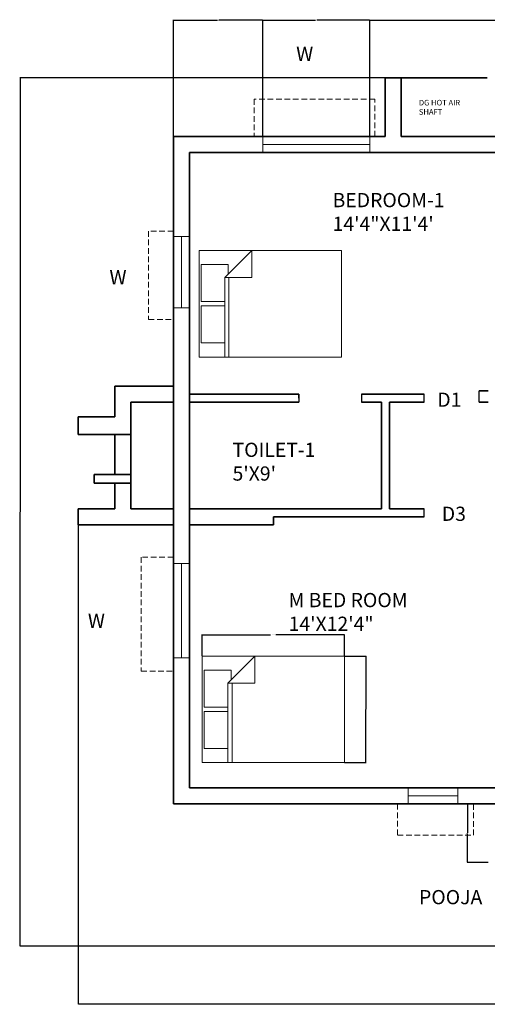
# Model space of a CAD drawing. Units: inches. Extents: x 514 to 1200, y -110 to 470.
# Tile 1 of 3: x 514 to 777, y -84 to 470. Entities that reach past the tile are written whole.
import ezdxf

# ---------------------------------------------------------------- set-up
doc = ezdxf.new("R2010")
doc.units = ezdxf.units.IN
doc.linetypes.add('HIDDEN2', pattern=[4.7625, 3.175, -1.5875])
for name, color, linetype, lineweight in [('A-ANNO-DIMS', 2, 'Continuous', 18), ('A-ANNO-IDEN', 3, 'Continuous', 18), ('A-AREA-IDEN', 7, 'Continuous', 18), ('A-DOOR', 3, 'Continuous', 25), ('A-FLOR-OVHD', 8, 'HIDDEN2', 18), ('A-FURN', 8, 'Continuous', 18), ('A-GLAZ', 4, 'Continuous', 18), ('A-WALL', 7, 'Continuous', 35)]:
    doc.layers.add(name, color=color, linetype=linetype, lineweight=lineweight)
doc.dimstyles.get("Standard").update_dxf_attribs({"dimtxt": 0.18, "dimasz": 0.18, "dimexe": 0.18, "dimexo": 0.0625, "dimgap": 0.09, "dimtad": 0, "dimtih": 1, "dimtoh": 1, "dimdec": 4, "dimzin": 0, "dimdsep": 46, "dimtxsty": 'Standard', "dimcen": 0.09, "dimadec": 0, "dimazin": 0, "dimtfac": 1, "dimtdec": 4, "dimtofl": 0, "dimtmove": 0, "dimatfit": 3, "dimfxl": 1, "dimtolj": 1, "dimtzin": 0, "dimarcsym": 0})

# ---------------------------------------------------------------- blocks, each defined once
blk = doc.blocks.new('Bed - Queen')
for p, q in [((0, -80.00003), (0, 0)), ((0, 0), (59.99999, 0)), ((59.99999, 0), (59.99999, -80.00003)), ((7.99999, -1.2), (28.79998, -1.2)), ((7.99999, -14.4), (7.99999, -1.2)), ((28.79998, -1.2), (28.79998, -14.4)), ((31.19999, -1.2), (51.99999, -1.2)), ((31.19999, -14.4), (31.19999, -1.2)), ((51.99999, -1.2), (51.99999, -16.4)), ((0, -14.4), (44.8, -14.4)), ((59.99999, -29.6), (44.8, -14.4)), ((44.8, -14.4), (44.8, -29.6)), ((51.99999, -16.4), (46.79936, -16.4)), ((44.8, -16.8), (0, -16.8)), ((44.8, -29.6), (59.99999, -29.6)), ((59.99999, -80.00003), (0, -80.00003))]:
    blk.add_line(p, q)
blk = doc.blocks.new('*D14')
at = {"layer": 'A-ANNO-DIMS', "color": 0, "lineweight": -2, "transparency": 16777216}
for p, q in [((617.04, 112.31), (617.04, 124.43)), ((617.22, 124.25), (655.52, 124.25)), ((696.86, 124.25), (658.55, 124.25)), ((697.04, 112.31), (697.04, 124.43))]:
    blk.add_line(p, q, dxfattribs=at)
at = {"layer": 'A-ANNO-DIMS', "color": 0, "transparency": 16777216}
for points in [[(617.22, 124.28), (617.22, 124.22), (617.04, 124.25)], [(696.86, 124.28), (696.86, 124.22), (697.04, 124.25)]]:
    blk.add_solid(points, dxfattribs=at)
at = {"layer": 'Defpoints', "color": 0, "transparency": 16777216}
for p in [(617.04, 124.25), (617.04, 112.25), (697.04, 112.25)]:
    blk.add_point(p, dxfattribs=at)
at = {"layer": 'A-ANNO-DIMS', "color": 0, "transparency": 16777216, "insert": (657.04, 124.25), "char_height": 0.18, "attachment_point": 5}
blk.add_mtext('\\A1;QUEEN BED 80 TYP.', dxfattribs=at)
blk = doc.blocks.new('*D15')
at = {"layer": 'A-ANNO-DIMS', "color": 0, "lineweight": -2, "transparency": 16777216}
for p, q in [((697.1, 112.25), (709.22, 112.25)), ((709.04, 112.07), (709.04, 82.43)), ((709.04, 52.43), (709.04, 82.07)), ((697.1, 52.25), (709.22, 52.25))]:
    blk.add_line(p, q, dxfattribs=at)
at = {"layer": 'A-ANNO-DIMS', "color": 0, "transparency": 16777216}
for points in [[(709.01, 112.07), (709.07, 112.07), (709.04, 112.25)], [(709.01, 52.43), (709.07, 52.43), (709.04, 52.25)]]:
    blk.add_solid(points, dxfattribs=at)
at = {"layer": 'Defpoints', "color": 0, "transparency": 16777216}
for p in [(697.04, 112.25), (709.04, 112.25), (697.04, 52.25)]:
    blk.add_point(p, dxfattribs=at)
at = {"layer": 'A-ANNO-DIMS', "color": 0, "transparency": 16777216, "insert": (709.04, 82.25), "char_height": 0.18, "attachment_point": 5}
blk.add_mtext('\\A1;60 TYP.', dxfattribs=at)
blk = doc.blocks.new('*D17')
at = {"layer": 'A-ANNO-DIMS', "color": 0, "lineweight": -2, "transparency": 16777216}
for p, q in [((777.83, 29.02), (766.01, 29.02)), ((766.19, 28.84), (766.19, 12.7)), ((766.19, -3.8), (766.19, 12.34)), ((777.83, -3.98), (766.01, -3.98))]:
    blk.add_line(p, q, dxfattribs=at)
at = {"layer": 'A-ANNO-DIMS', "color": 0, "transparency": 16777216}
for points in [[(766.16, 28.84), (766.22, 28.84), (766.19, 29.02)], [(766.16, -3.8), (766.22, -3.8), (766.19, -3.98)]]:
    blk.add_solid(points, dxfattribs=at)
at = {"layer": 'Defpoints', "color": 0, "transparency": 16777216}
for p in [(766.19, 29.02), (777.89, 29.02), (777.89, -3.98)]:
    blk.add_point(p, dxfattribs=at)
at = {"layer": 'A-ANNO-DIMS', "color": 0, "transparency": 16777216, "insert": (766.19, 12.52), "char_height": 0.18, "attachment_point": 5}
blk.add_mtext('\\A1;33 TYP.', dxfattribs=at)
blk = doc.blocks.new('*D24')
at = {"layer": 'A-ANNO-DIMS', "color": 0, "lineweight": -2, "transparency": 16777216}
for p, q in [((600.890564, 404.583196), (600.890564, 470.250696)), ((601.070564, 470.070696), (625.592556, 470.070696)), ((650.924548, 470.070696), (626.402556, 470.070696)), ((651.104548, 404.583196), (651.104548, 470.250696))]:
    blk.add_line(p, q, dxfattribs=at)
at = {"layer": 'A-ANNO-DIMS', "color": 0, "transparency": 16777216}
for points in [[(601.070564, 470.100696), (601.070564, 470.040696), (600.890564, 470.070696)], [(650.924548, 470.100696), (650.924548, 470.040696), (651.104548, 470.070696)]]:
    blk.add_solid(points, dxfattribs=at)
at = {"layer": 'Defpoints', "color": 0, "transparency": 16777216}
for p in [(651.104548, 470.070696), (600.890564, 404.520696), (651.104548, 404.520696)]:
    blk.add_point(p, dxfattribs=at)
at = {"layer": 'A-ANNO-DIMS', "color": 0, "transparency": 16777216, "insert": (625.997556, 470.070696), "char_height": 0.18, "attachment_point": 5}
blk.add_mtext('\\A1;50.21', dxfattribs=at)
blk = doc.blocks.new('*D25')
at = {"layer": 'A-ANNO-DIMS', "color": 0, "lineweight": -2, "transparency": 16777216}
for p, q in [((651.1, 404.58), (651.1, 470.25)), ((651.28, 470.07), (680.79, 470.07)), ((711.1, 470.07), (681.6, 470.07)), ((711.28, 404.58), (711.28, 470.25))]:
    blk.add_line(p, q, dxfattribs=at)
at = {"layer": 'A-ANNO-DIMS', "color": 0, "transparency": 16777216}
for points in [[(651.28, 470.1), (651.28, 470.04), (651.1, 470.07)], [(711.1, 470.1), (711.1, 470.04), (711.28, 470.07)]]:
    blk.add_solid(points, dxfattribs=at)
at = {"layer": 'Defpoints', "color": 0, "transparency": 16777216}
for p in [(711.28, 470.07), (651.1, 404.52), (711.28, 404.52)]:
    blk.add_point(p, dxfattribs=at)
at = {"layer": 'A-ANNO-DIMS', "color": 0, "transparency": 16777216, "insert": (681.19, 470.07), "char_height": 0.18, "attachment_point": 5}
blk.add_mtext('\\A1;60.18', dxfattribs=at)
blk = doc.blocks.new('*D26')
at = {"layer": 'A-ANNO-DIMS', "color": 0, "lineweight": -2, "transparency": 16777216}
for p, q in [((711.28, 404.58), (711.28, 470.25)), ((711.46, 470.07), (797.69, 470.07)), ((884.94, 470.07), (798.71, 470.07)), ((885.12, 404.58), (885.12, 470.25))]:
    blk.add_line(p, q, dxfattribs=at)
at = {"layer": 'A-ANNO-DIMS', "color": 0, "transparency": 16777216}
for points in [[(711.46, 470.1), (711.46, 470.04), (711.28, 470.07)], [(884.94, 470.1), (884.94, 470.04), (885.12, 470.07)]]:
    blk.add_solid(points, dxfattribs=at)
at = {"layer": 'Defpoints', "color": 0, "transparency": 16777216}
for p in [(885.12, 470.07), (711.28, 404.52), (885.12, 404.52)]:
    blk.add_point(p, dxfattribs=at)
at = {"layer": 'A-ANNO-DIMS', "color": 0, "transparency": 16777216, "insert": (798.2, 470.07), "char_height": 0.18, "attachment_point": 5}
blk.add_mtext('\\A1;173.83', dxfattribs=at)
blk = doc.blocks.new('*D36')
at = {"layer": 'A-ANNO-DIMS', "color": 0, "lineweight": -2, "transparency": 16777216}
for p, q in [((1166.99, 243.01), (1166.99, -83.71)), ((547.32, 185.96), (547.32, -83.71)), ((547.5, -83.53), (856.73, -83.53)), ((1166.81, -83.53), (857.57, -83.53))]:
    blk.add_line(p, q, dxfattribs=at)
at = {"layer": 'A-ANNO-DIMS', "color": 0, "transparency": 16777216}
for points in [[(547.5, -83.5), (547.5, -83.56), (547.32, -83.53)], [(1166.81, -83.5), (1166.81, -83.56), (1166.99, -83.53)]]:
    blk.add_solid(points, dxfattribs=at)
at = {"layer": 'Defpoints', "color": 0, "transparency": 16777216}
for p in [(1166.99, 243.07), (547.32, 186.02), (1166.99, -83.53)]:
    blk.add_point(p, dxfattribs=at)
at = {"layer": 'A-ANNO-DIMS', "color": 0, "transparency": 16777216, "insert": (857.15, -83.53), "char_height": 0.18, "attachment_point": 5}
blk.add_mtext('\\A1;619.7', dxfattribs=at)
blk = doc.blocks.new('*D37')
at = {"layer": 'A-ANNO-DIMS', "color": 0, "lineweight": -2, "transparency": 16777216}
for p, q in [((719.82324, 437.520696), (514.588716, 437.520696)), ((514.768716, 437.340696), (514.768716, 193.450696)), ((514.768716, -50.799304), (514.768716, 193.090696)), ((846.828064, -50.979304), (514.588716, -50.979304))]:
    blk.add_line(p, q, dxfattribs=at)
at = {"layer": 'A-ANNO-DIMS', "color": 0, "transparency": 16777216}
for points in [[(514.738716, 437.340696), (514.798716, 437.340696), (514.768716, 437.520696)], [(514.738716, -50.799304), (514.798716, -50.799304), (514.768716, -50.979304)]]:
    blk.add_solid(points, dxfattribs=at)
at = {"layer": 'Defpoints', "color": 0, "transparency": 16777216}
for p in [(514.768716, 437.520696), (719.88574, 437.520696), (846.890564, -50.979304)]:
    blk.add_point(p, dxfattribs=at)
at = {"layer": 'A-ANNO-DIMS', "color": 0, "transparency": 16777216, "insert": (514.768716, 193.270696), "char_height": 0.18, "attachment_point": 5}
blk.add_mtext('\\A1;488.5', dxfattribs=at)

msp = doc.modelspace()

# ---------------------------------------------------------------- linework, layer by layer
at = {"layer": 'A-DOOR'}
for p, q in [((772.9065, 255.0207), (772.9065, 261.4252)), ((671.3734, 257.2707), (671.3734, 259.5207)), ((671.3734, 259.5207), (671.3734, 255.0207)), ((706.6585, 259.5207), (706.6585, 255.0207)), ((741.8906, 255.0207), (741.8906, 259.5207)), ((741.8906, 190.5207), (741.8906, 195.0207))]:
    msp.add_line(p, q, dxfattribs=at)
at = {"layer": 'A-FLOR-OVHD'}
for p, q in [((714.1676, 425.5708), (646.3079, 425.5708)), ((646.3079, 425.5708), (646.3079, 404.5207)), ((714.1676, 404.5207), (714.1676, 425.5708)), ((600.8906, 351.2891), (586.9342, 351.2891)), ((586.9342, 351.2891), (586.9342, 301.4805)), ((586.9342, 301.4805), (600.8906, 301.4805)), ((600.8906, 167.7812), (582.8053, 167.7812)), ((582.8053, 167.7812), (582.8053, 103.6598)), ((582.8053, 103.6598), (600.8906, 103.6598)), ((726.9376, 29.0207), (726.9376, 11.4444)), ((769.6276, 11.4444), (769.6276, 29.0207)), ((726.9376, 11.4444), (769.6276, 11.4444))]:
    msp.add_line(p, q, dxfattribs=at)
at = {"layer": 'A-GLAZ'}
for p, q in [((651.1045, 404.5207), (651.1045, 395.5207)), ((711.283, 400.0207), (711.283, 404.5207)), ((711.283, 404.5207), (711.283, 395.5207)), ((651.1045, 395.5207), (651.1045, 400.0207)), ((651.1045, 400.0207), (711.283, 400.0207)), ((600.8906, 348.2213), (609.8906, 348.2213)), ((609.8906, 348.2213), (605.3906, 348.2213)), ((605.3906, 348.2213), (605.3906, 308.2207)), ((605.3906, 308.2207), (600.8906, 308.2207)), ((600.8906, 308.2207), (609.8906, 308.2207)), ((600.8906, 164.3544), (609.8906, 164.3544)), ((609.8906, 164.3544), (605.3906, 164.3544)), ((605.3906, 164.3544), (605.3906, 111.1618)), ((605.3906, 111.1618), (600.8906, 111.1618)), ((600.8906, 111.1618), (609.8906, 111.1618)), ((732.8501, 38.0207), (732.8501, 29.0207)), ((732.8501, 29.0207), (732.8501, 33.5207)), ((732.8501, 33.5207), (760.8245, 33.5207)), ((760.8245, 33.5207), (760.8245, 38.0207)), ((760.8245, 38.0207), (760.8245, 29.0207))]:
    msp.add_line(p, q, dxfattribs=at)
at = {"layer": 'A-WALL'}
for p, q in [((719.8857, 437.5207), (719.8857, 404.5207)), ((728.8857, 437.5207), (719.8857, 437.5207)), ((777.3906, 437.5207), (728.8857, 437.5207)), ((728.8857, 437.5207), (728.8857, 404.5207)), ((600.8906, 404.5207), (719.8857, 404.5207)), ((600.8906, 29.0207), (600.8906, 404.5207)), ((728.8857, 404.5207), (1142.8906, 404.5207)), ((609.8906, 395.5207), (781.8906, 395.5207)), ((609.8906, 38.0207), (609.8906, 395.5207)), ((567.8906, 264.0207), (567.8906, 246.7778)), ((600.8906, 264.0207), (567.8906, 264.0207)), ((772.9065, 261.4252), (777.8906, 261.4252)), ((600.8906, 255.0207), (576.8906, 255.0207)), ((576.8906, 255.0207), (576.8906, 195.0207)), ((609.8906, 259.5207), (671.3734, 259.5207)), ((609.8906, 259.5207), (671.3734, 259.5207)), ((609.8906, 255.0207), (671.3734, 255.0207)), ((609.8906, 255.0207), (671.3734, 255.0207)), ((706.6585, 259.5207), (741.8906, 259.5207)), ((706.6585, 259.5207), (741.8906, 259.5207)), ((706.6585, 255.0207), (717.8906, 255.0207)), ((706.6585, 255.0207), (717.8906, 255.0207)), ((717.8906, 195.0207), (717.8906, 255.0207)), ((722.3906, 195.0207), (722.3906, 255.0207)), ((722.3906, 255.0207), (741.8906, 255.0207)), ((722.3906, 255.0207), (741.8906, 255.0207)), ((777.8906, 255.0207), (772.9065, 255.0207)), ((547.3187, 236.9335), (547.3187, 246.7778)), ((547.3187, 246.7778), (567.8906, 246.7778)), ((576.8906, 236.9335), (547.3187, 236.9335)), ((567.8906, 236.9335), (567.8906, 214.3425)), ((576.8906, 214.3425), (556.4172, 214.3425)), ((556.4172, 214.3425), (556.4172, 209.4406)), ((556.4172, 209.4406), (576.8906, 209.4406)), ((567.8906, 209.4406), (567.8906, 195.0207)), ((547.3187, 186.0207), (547.3187, 195.0207)), ((547.3187, 195.0207), (567.8906, 195.0207)), ((576.8906, 195.0207), (600.8906, 195.0207)), ((609.8906, 195.0207), (717.8906, 195.0207)), ((722.3906, 195.0207), (741.8906, 195.0207)), ((657.1918, 186.0207), (657.1918, 190.5207)), ((657.1918, 190.5207), (722.3906, 190.5207)), ((657.1918, 190.5207), (741.8906, 190.5207)), ((567.8906, 186.0207), (547.3187, 186.0207)), ((567.8906, 186.0207), (600.8906, 186.0207)), ((609.8906, 186.0207), (657.1918, 186.0207)), ((609.8906, 38.0207), (983.8906, 38.0207)), ((600.8906, 29.0207), (983.8906, 29.0207))]:
    msp.add_line(p, q, dxfattribs=at)

# ---------------------------------------------------------------- block references
at = {"layer": 'A-FURN', "rotation": 90}
for p in [(615.3484, 280.4737), (617.0399, 52.2514)]:
    msp.add_blockref('Bed - Queen', p, dxfattribs=at)

# ---------------------------------------------------------------- texts
at = {"layer": 'A-ANNO-IDEN', "char_height": 8, "attachment_point": 1}
for s, insert in [('{\\fTimes New Roman|b0|i0|c0|p18;W}', (669.9162, 455.055)), ('{\\fTimes New Roman|b0|i0|c0|p18;W}', (564.9379, 329.3302)), ('{\\fTimes New Roman|b0|i0|c0|p18;D1}', (749.2884, 260.4506)), ('\\pxt2;{\\fTimes New Roman|b0|i0|c0|p18;D3}', (751.8117, 196.2713)), ('{\\fTimes New Roman|b0|i0|c0|p18;W}', (552.8049, 136.0875))]:
    msp.add_mtext_dynamic_manual_height_columns(s, width=92.773282, gutter_width=12.5, heights=[0], dxfattribs=dict(at, insert=insert))
at = {"layer": 'A-AREA-IDEN', "attachment_point": 1}
for s, width, gutter_width, insert, char_height in [('{\\fTimes New Roman|b0|i0|c0|p18;DG HOT AIR SHAFT}', 36.387649, 4.9028, (738.9027, 425.1429), 3.13777), ('{\\fTimes New Roman|b0|i0|c0|p18;BEDROOM-1\\P14\'4"X11\'4\'}', 92.773282, 12.5, (690.384, 372.7481), 8), ("{\\fTimes New Roman|b0|i0|c0|p18;TOILET-1\\P5'X9'}", 92.773282, 12.5, (634.1481, 232.2526), 8), ('{\\fTimes New Roman|b0|i0|c0|p18;M BED ROOM\\P14\'X12\'4"}', 92.773282, 12.5, (665.6831, 147.7235), 8), ('{\\fTimes New Roman|b0|i0|c0|p18;POOJA}', 92.773282, 12.5, (739.0036, -19.4159), 8)]:
    msp.add_mtext_dynamic_manual_height_columns(s, width=width, gutter_width=gutter_width, heights=[0], dxfattribs=dict(at, insert=insert, char_height=char_height))

# ---------------------------------------------------------------- dimensions: what is measured, and where the dimension line sits
at = {"layer": 'A-ANNO-DIMS'}
for base, p1, p2, override, picture, middle in [((651.1045, 470.0707), (600.8906, 404.5207), (651.1045, 404.5207), {"dimdec": 2, "dimlfac": 1, "dimrnd": 0, "dimzin": 0, "dimdsep": 46, "dimlunit": 2}, '*D24', (625.9976, 470.0707)), ((711.283, 470.0707), (651.1045, 404.5207), (711.283, 404.5207), {"dimdec": 2, "dimlfac": 1, "dimrnd": 0, "dimzin": 0, "dimdsep": 46, "dimlunit": 2}, '*D25', (681.1938, 470.0707)), ((885.1179, 470.0707), (711.283, 404.5207), (885.1179, 404.5207), {"dimdec": 2, "dimlfac": 1, "dimrnd": 0, "dimzin": 0, "dimdsep": 46, "dimlunit": 2}, '*D26', (798.2005, 470.0707)), ((1166.9893, -83.5293), (547.3187, 186.0207), (1166.9893, 243.0707), {"dimdec": 1, "dimlfac": 1, "dimrnd": 0, "dimzin": 0, "dimdsep": 46, "dimlunit": 2}, '*D36', (857.154, -83.5293))]:
    dim = msp.add_linear_dim(base=base, p1=p1, p2=p2, dimstyle='Standard', override=override, dxfattribs=at)
    dim.commit()
    dim.dimension.update_dxf_attribs({"geometry": picture, "text_midpoint": middle})
dim = msp.add_linear_dim(base=(514.7687, 437.5207), p1=(846.8906, -50.9793), p2=(719.8857, 437.5207), angle=90, dimstyle='Standard', override={"dimdec": 1, "dimlfac": 1, "dimrnd": 0, "dimzin": 0, "dimdsep": 46, "dimlunit": 2}, dxfattribs=at)
dim.commit()
dim.dimension.update_dxf_attribs({"geometry": '*D37', "text_midpoint": (514.7687, 193.2707)})
for base, p1, p2, angle, text, picture, middle in [((617.0399, 124.2514), (697.0399, 112.2514), (617.0399, 112.2514), 180, 'QUEEN BED <> TYP.', '*D14', (657.0399, 124.2514)), ((709.0399, 112.2514), (697.0399, 52.2514), (697.0399, 112.2514), 90, '<> TYP.', '*D15', (709.0399, 82.2514)), ((766.1906, 29.0207), (777.8906, -3.9793), (777.8906, 29.0207), 90, '<> TYP.', '*D17', (766.1906, 12.5207))]:
    dim = msp.add_linear_dim(base=base, p1=p1, p2=p2, angle=angle, text=text, dimstyle='Standard', override={"dimdec": 0, "dimlfac": 1, "dimrnd": 0, "dimzin": 0, "dimdsep": 46, "dimlunit": 2}, dxfattribs=at)
    dim.commit()
    dim.dimension.update_dxf_attribs({"geometry": picture, "text_midpoint": middle})

doc.saveas('drawing.dxf')
